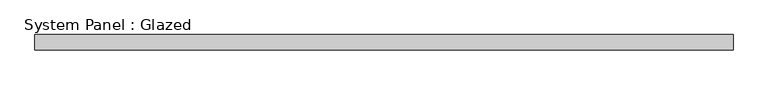
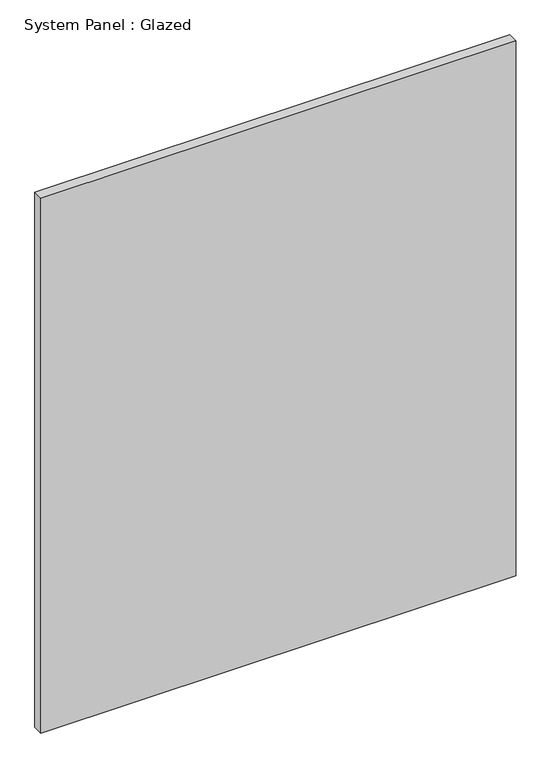
"""IFC4 building model written with IfcOpenShell, lengths in millimetres: plate geometry, System Panel : Glazed."""

from ifc_helpers import new_model, si_unit, origin, origin_with_axes, place, context, project, spatial, polyline, outline, extrude, source, transform, mapped, element, save


def system_panel_glazed_19ddc366(model_context):
    return source(origin(), model_context, "Body", "SweptSolid", [
        extrude(outline(polyline([(580.39, 19.05), (-580.39, 19.05), (-580.39, 44.45), (580.39, 44.45), (580.39, 19.05)])), origin_with_axes(), (0.0, 0.0, 1.0), 1382.6020555),
    ])


if __name__ == "__main__":
    model = new_model("IFC4")
    model_context = context("Model", 3, world=origin())
    ifc_project = project(units=[si_unit("LENGTHUNIT", "METRE", prefix="MILLI")], contexts=[model_context])
    site = spatial("IfcSite", under=ifc_project)
    building = spatial("IfcBuilding", under=site)
    placement = place(None, origin())
    system_panel_glazed_shape = system_panel_glazed_19ddc366(model_context)
    element("IfcPlate", 1, ObjectType="System Panel : Glazed", at=placement, inside=building, context=model_context, shape_type="MappedRepresentation", body=[
        mapped(system_panel_glazed_shape, transform((0.0, 0.0, 0.0), x_axis=(1.0, 0.0, 0.0), y_axis=(0.0, 1.0, 0.0), z_axis=(0.0, 0.0, 1.0))),
    ])
    save(model, "model.ifc")

# Revit data of these elements
# Type "System Panel : Glazed"
#   Construction Type Id = "GSP4R"
#   Analytic Construction = "1/8 in Pilkington single glazing"
#   Visual Light Transmittance = 0.9
#   Solar Heat Gain Coefficient = 0.86
#   Heat Transfer Coefficient (U) = 1.18115 BTU/(h·ft²·°F)
#   Define Thermal Properties by = 1
# Element 1 (IfcPlate, "System Panel : Glazed")
#   Materials on its faces: "Glass"
# Materials
#   "Glass": class "Glass", colour RGB 0 128 192, transparency 0.75, Description = "Soda Lime Glass", Cost = 0
